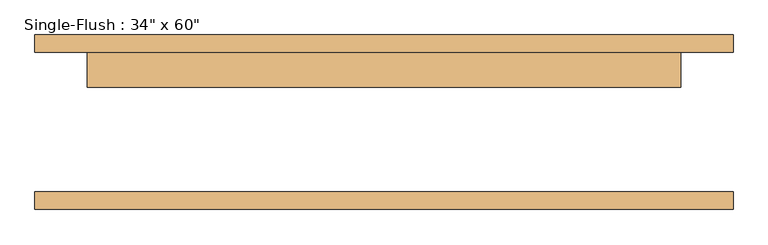
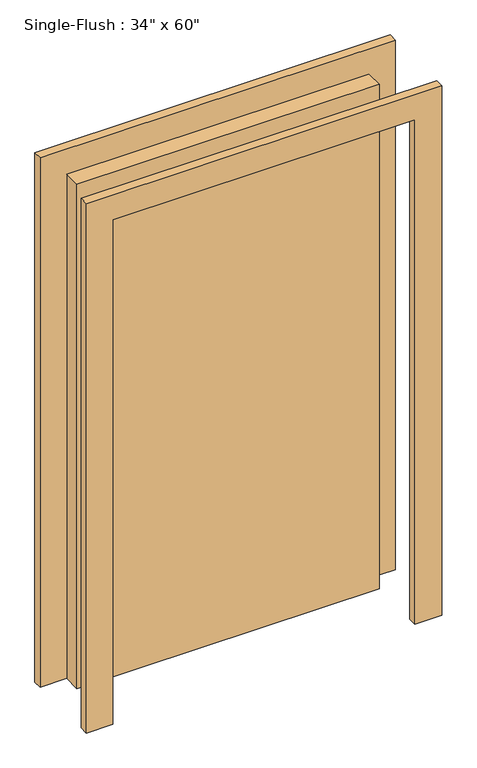
"""IFC4 building model written with IfcOpenShell, lengths in millimetres: door geometry."""

from ifc_helpers import new_model, si_unit, frame, origin, origin_with_axes, place, context, project, spatial, polyline, outline, extrude, source, transform, mapped, element, save


def door_3e6ab620(model_context):
    return source(origin(), model_context, "Body", "SweptSolid", [
        extrude(outline(polyline([(1600.2, -508.0), (0.0, -508.0), (0.0, -431.8), (1524.0, -431.8), (1524.0, 431.8), (0.0, 431.8), (0.0, 508.0), (1600.2, 508.0), (1600.2, -508.0)])), frame((0.0, 101.6, 0.0), z_axis=(0.0, 1.0, 0.0), x_axis=(0.0, 0.0, 1.0)), (0.0, 0.0, 1.0), 25.4),
        extrude(outline(polyline([(1600.2, 508.0), (1600.2, -508.0), (0.0, -508.0), (0.0, -431.8), (1524.0, -431.8), (1524.0, 431.8), (0.0, 431.8), (0.0, 508.0), (1600.2, 508.0)])), frame((0.0, -127.0, 0.0), z_axis=(0.0, 1.0, 0.0), x_axis=(0.0, 0.0, 1.0)), (0.0, 0.0, 1.0), 25.4),
        extrude(outline(polyline([(431.8, 50.8), (-431.8, 50.8), (-431.8, 101.6), (431.8, 101.6), (431.8, 50.8)])), origin_with_axes(), (0.0, 0.0, 1.0), 1524.0),
    ])


if __name__ == "__main__":
    model = new_model("IFC4")
    model_context = context("Model", 3, world=origin())
    ifc_project = project(units=[si_unit("LENGTHUNIT", "METRE", prefix="MILLI")], contexts=[model_context])
    site = spatial("IfcSite", under=ifc_project)
    building = spatial("IfcBuilding", under=site)
    placement = place(None, origin())
    door_shape = door_3e6ab620(model_context)
    element("IfcDoor", 1, ObjectType="Single-Flush : 34\" x 60\"", at=placement, inside=building, context=model_context, shape_type="MappedRepresentation", body=[
        mapped(door_shape, transform((0.0, 0.0, 0.0), x_axis=(1.0, 0.0, 0.0), y_axis=(0.0, 1.0, 0.0), z_axis=(0.0, 0.0, 1.0))),
    ])
    save(model, "model.ifc")

# Revit data of these elements
# Type "Single-Flush : 34\" x 60\""
#   Type Mark = "8"
#   Construction Type Id = "MDOOR"
#   Assembly Code = "C1020"
#   Analytic Construction = "Metal"
#   Thickness = 0' - 2"
#   Heat Transfer Coefficient (U) = 0.651978 BTU/(h·ft²·°F)
#   Height = 5' - 0"
#   Trim Projection Ext = 0' - 1"
#   Trim Projection Int = 0' - 1"
#   Trim Width = 0' - 3"
#   Width = 2' - 10"
#   Define Thermal Properties by = 1
#   Door Material = Door - Panel
#   Frame Material = Door - Frame
#   Visual Light Transmittance = 0
#   Solar Heat Gain Coefficient = 0
#   Function = (empty or 0)
#   Wall Closure = (empty or 0)
# Element 1 (IfcDoor, "Single-Flush : 34\" x 60\"")
#   Materials on its faces: "Door - Frame", "Door - Panel"
# Materials
#   "Door - Panel": class "Wood", colour RGB 210 159 95, transparency 0
#   "Door - Frame": colour RGB 118 70 51, transparency 0
